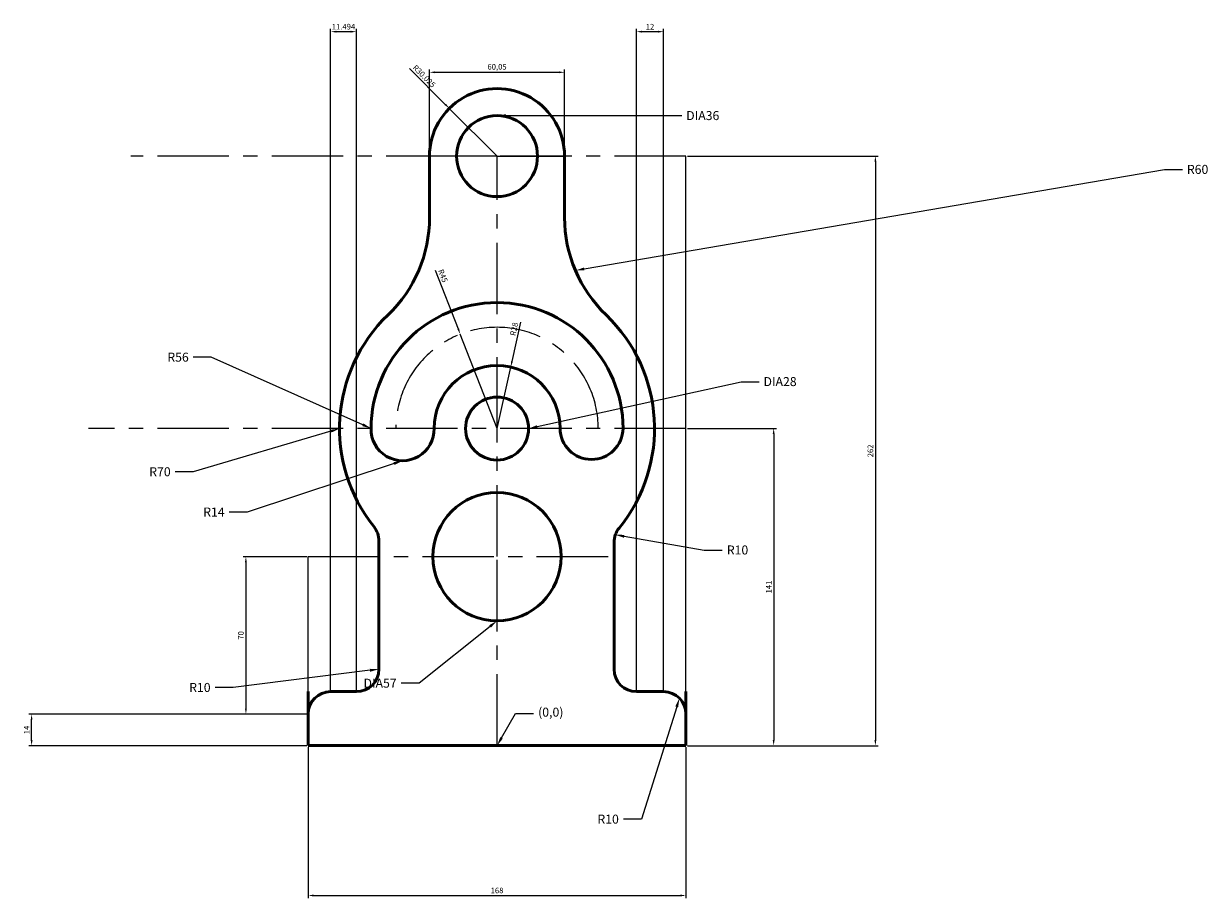
# Model space of a CAD drawing. Units: millimetres. Extents: x 2245 to 2771, y 1191 to 1580.
import ezdxf
from ezdxf import colors
from ezdxf.entities.mleader import LeaderData, LeaderLine
from ezdxf.math import Vec2, Vec3

# ---------------------------------------------------------------- set-up
doc = ezdxf.new("R2010")
doc.units = ezdxf.units.MM
doc.linetypes.add('CENTER', pattern=[50.8, 31.75, -6.35, 6.35, -6.35])
for name, color, linetype, lineweight in [('M-CNTR', 4, 'CENTER', 18), ('M-CONS', 8, 'Continuous', 13), ('M-DIMS', 2, 'Continuous', 25), ('M-OUTL', 7, 'Continuous', 50), ('M-TEXT', 7, 'Continuous', 25)]:
    doc.layers.add(name, color=color, linetype=linetype, lineweight=lineweight)
doc.styles.get("Standard").update_dxf_attribs({"font": 'arial.ttf'})
doc.dimstyles.new('ISO-25', dxfattribs={"dimtxt": 2.5, "dimasz": 2.5, "dimexe": 1.25, "dimexo": 0.625, "dimtad": 1, "dimtxsty": 'Standard', "dimcen": 2.5, "dimadec": 0, "dimazin": 0, "dimtfac": 1, "dimtmove": 0, "dimatfit": 3, "dimfxl": 1, "dimarcsym": 0})

# ---------------------------------------------------------------- blocks, each defined once
blk = doc.blocks.new('*D1')
at = {"layer": 'Defpoints', "color": 0, "transparency": 16777216}
for p in [(2485.25, 1558.14), (2425.2, 1520.84), (2485.25, 1520.87)]:
    blk.add_point(p, dxfattribs=at)
at = {"layer": 'M-DIMS', "color": 0, "lineweight": -2, "transparency": 16777216}
for p, q in [((2425.2, 1521.47), (2425.2, 1559.39)), ((2485.25, 1521.5), (2485.25, 1559.39)), ((2427.7, 1558.14), (2482.75, 1558.14))]:
    blk.add_line(p, q, dxfattribs=at)
at = {"layer": 'M-DIMS', "color": 0, "transparency": 16777216}
for points in [[(2427.7, 1558.56), (2427.7, 1557.73), (2425.2, 1558.14)], [(2482.75, 1558.56), (2482.75, 1557.73), (2485.25, 1558.14)]]:
    blk.add_solid(points, dxfattribs=at)
at = {"layer": 'M-DIMS', "color": 0, "transparency": 16777216, "insert": (2455.23, 1560.27), "char_height": 2.5, "attachment_point": 5}
blk.add_mtext('60,05', dxfattribs=at)
blk = doc.blocks.new('*D2')
at = {"layer": 'Defpoints', "color": 0, "transparency": 16777216}
for p in [(2539.23, 1520.87), (2539.23, 1258.87), (2623.43, 1258.87)]:
    blk.add_point(p, dxfattribs=at)
at = {"layer": 'M-DIMS', "color": 0, "lineweight": -2, "transparency": 16777216}
for p, q in [((2539.85, 1520.87), (2624.68, 1520.87)), ((2623.43, 1518.37), (2623.43, 1261.37)), ((2539.85, 1258.87), (2624.68, 1258.87))]:
    blk.add_line(p, q, dxfattribs=at)
at = {"layer": 'M-DIMS', "color": 0, "transparency": 16777216}
for points in [[(2623.01, 1518.37), (2623.85, 1518.37), (2623.43, 1520.87)], [(2623.01, 1261.37), (2623.85, 1261.37), (2623.43, 1258.87)]]:
    blk.add_solid(points, dxfattribs=at)
at = {"layer": 'M-DIMS', "color": 0, "transparency": 16777216, "insert": (2621.53, 1389.87), "char_height": 2.5, "attachment_point": 5, "rotation": 90}
blk.add_mtext('262', dxfattribs=at)
blk = doc.blocks.new('*D3')
at = {"layer": 'Defpoints', "color": 0, "transparency": 16777216}
for p in [(2371.23, 1342.87), (2343.58, 1272.87), (2371.23, 1272.87)]:
    blk.add_point(p, dxfattribs=at)
at = {"layer": 'M-DIMS', "color": 0, "lineweight": -2, "transparency": 16777216}
for p, q in [((2370.6, 1342.87), (2342.33, 1342.87)), ((2343.58, 1340.37), (2343.58, 1275.37)), ((2370.6, 1272.87), (2342.33, 1272.87))]:
    blk.add_line(p, q, dxfattribs=at)
at = {"layer": 'M-DIMS', "color": 0, "transparency": 16777216}
for points in [[(2343.17, 1340.37), (2344, 1340.37), (2343.58, 1342.87)], [(2343.17, 1275.37), (2344, 1275.37), (2343.58, 1272.87)]]:
    blk.add_solid(points, dxfattribs=at)
at = {"layer": 'M-DIMS', "color": 0, "transparency": 16777216, "insert": (2341.68, 1307.87), "char_height": 2.5, "attachment_point": 5, "rotation": 90}
blk.add_mtext('70', dxfattribs=at)
blk = doc.blocks.new('*D4')
at = {"layer": 'Defpoints', "color": 0, "transparency": 16777216}
for p in [(2539.23, 1399.87), (2539.23, 1258.87), (2578.21, 1258.87)]:
    blk.add_point(p, dxfattribs=at)
at = {"layer": 'M-DIMS', "color": 0, "lineweight": -2, "transparency": 16777216}
for p, q in [((2539.85, 1399.87), (2579.46, 1399.87)), ((2578.21, 1397.37), (2578.21, 1261.37)), ((2539.85, 1258.87), (2579.46, 1258.87))]:
    blk.add_line(p, q, dxfattribs=at)
at = {"layer": 'M-DIMS', "color": 0, "transparency": 16777216}
for points in [[(2577.79, 1397.37), (2578.62, 1397.37), (2578.21, 1399.87)], [(2577.79, 1261.37), (2578.62, 1261.37), (2578.21, 1258.87)]]:
    blk.add_solid(points, dxfattribs=at)
at = {"layer": 'M-DIMS', "color": 0, "transparency": 16777216, "insert": (2576.33, 1329.37), "char_height": 2.5, "attachment_point": 5, "rotation": 90}
blk.add_mtext('141', dxfattribs=at)
blk = doc.blocks.new('*D5')
at = {"layer": 'Defpoints', "color": 0, "transparency": 16777216}
for p in [(2371.23, 1258.87), (2539.23, 1258.87), (2539.23, 1192.29)]:
    blk.add_point(p, dxfattribs=at)
at = {"layer": 'M-DIMS', "color": 0, "lineweight": -2, "transparency": 16777216}
for p, q in [((2371.23, 1258.25), (2371.23, 1191.04)), ((2539.23, 1258.25), (2539.23, 1191.04)), ((2373.73, 1192.29), (2536.73, 1192.29))]:
    blk.add_line(p, q, dxfattribs=at)
at = {"layer": 'M-DIMS', "color": 0, "transparency": 16777216}
for points in [[(2373.73, 1192.7), (2373.73, 1191.87), (2371.23, 1192.29)], [(2536.73, 1192.7), (2536.73, 1191.87), (2539.23, 1192.29)]]:
    blk.add_solid(points, dxfattribs=at)
at = {"layer": 'M-DIMS', "color": 0, "transparency": 16777216, "insert": (2455.23, 1194.19), "char_height": 2.5, "attachment_point": 5}
blk.add_mtext('168', dxfattribs=at)
blk = doc.blocks.new('*D6')
at = {"layer": 'Defpoints', "color": 0, "transparency": 16777216}
for p in [(2248.31, 1272.87), (2371.23, 1272.87), (2371.23, 1258.87)]:
    blk.add_point(p, dxfattribs=at)
at = {"layer": 'M-DIMS', "color": 0, "lineweight": -2, "transparency": 16777216}
for p, q in [((2370.6, 1272.87), (2247.06, 1272.87)), ((2248.31, 1261.37), (2248.31, 1270.37)), ((2370.6, 1258.87), (2247.06, 1258.87))]:
    blk.add_line(p, q, dxfattribs=at)
at = {"layer": 'M-DIMS', "color": 0, "transparency": 16777216}
for points in [[(2247.9, 1270.37), (2248.73, 1270.37), (2248.31, 1272.87)], [(2247.9, 1261.37), (2248.73, 1261.37), (2248.31, 1258.87)]]:
    blk.add_solid(points, dxfattribs=at)
at = {"layer": 'M-DIMS', "color": 0, "transparency": 16777216, "insert": (2246.43, 1265.87), "char_height": 2.5, "attachment_point": 5, "rotation": 90}
blk.add_mtext('14', dxfattribs=at)
blk = doc.blocks.new('*D7')
at = {"layer": 'Defpoints', "color": 0, "transparency": 16777216}
for p in [(2392.72, 1576.2), (2381.23, 1282.87), (2392.72, 1282.87)]:
    blk.add_point(p, dxfattribs=at)
at = {"layer": 'M-DIMS', "color": 0, "lineweight": -2, "transparency": 16777216}
for p, q in [((2381.23, 1283.5), (2381.23, 1577.45)), ((2383.73, 1576.2), (2390.22, 1576.2)), ((2392.72, 1283.5), (2392.72, 1577.45))]:
    blk.add_line(p, q, dxfattribs=at)
at = {"layer": 'M-DIMS', "color": 0, "transparency": 16777216}
for points in [[(2383.73, 1576.62), (2383.73, 1575.78), (2381.23, 1576.2)], [(2390.22, 1576.62), (2390.22, 1575.78), (2392.72, 1576.2)]]:
    blk.add_solid(points, dxfattribs=at)
at = {"layer": 'M-DIMS', "color": 0, "transparency": 16777216, "insert": (2386.97, 1578.1), "char_height": 2.5, "attachment_point": 5}
blk.add_mtext('11.494', dxfattribs=at)
blk = doc.blocks.new('*D8')
at = {"layer": 'Defpoints', "color": 0, "transparency": 16777216}
for p in [(2529.23, 1576.2), (2517.23, 1282.87), (2529.23, 1282.87)]:
    blk.add_point(p, dxfattribs=at)
at = {"layer": 'M-DIMS', "color": 0, "lineweight": -2, "transparency": 16777216}
for p, q in [((2517.23, 1283.5), (2517.23, 1577.45)), ((2519.73, 1576.2), (2526.73, 1576.2)), ((2529.23, 1283.5), (2529.23, 1577.45))]:
    blk.add_line(p, q, dxfattribs=at)
at = {"layer": 'M-DIMS', "color": 0, "transparency": 16777216}
for points in [[(2519.73, 1576.62), (2519.73, 1575.78), (2517.23, 1576.2)], [(2526.73, 1576.62), (2526.73, 1575.78), (2529.23, 1576.2)]]:
    blk.add_solid(points, dxfattribs=at)
at = {"layer": 'M-DIMS', "color": 0, "transparency": 16777216, "insert": (2523.23, 1578.08), "char_height": 2.5, "attachment_point": 5}
blk.add_mtext('12', dxfattribs=at)
blk = doc.blocks.new('*D9')
at = {"layer": 'Defpoints', "color": 0, "transparency": 16777216}
for p in [(2461.3, 1427.13), (2455.23, 1399.8)]:
    blk.add_point(p, dxfattribs=at)
at = {"layer": 'M-DIMS', "color": 0, "lineweight": -2, "transparency": 16777216}
for p, q in [((2465.73, 1447.06), (2461.84, 1429.57)), ((2455.23, 1399.8), (2461.3, 1427.13))]:
    blk.add_line(p, q, dxfattribs=at)
at = {"layer": 'M-DIMS', "color": 0, "transparency": 16777216}
blk.add_solid([(2461.44, 1429.66), (2462.25, 1429.48), (2461.3, 1427.13)], dxfattribs=at)
at = {"layer": 'M-DIMS', "color": 0, "transparency": 16777216, "insert": (2463.09, 1443.94), "char_height": 2.5, "attachment_point": 5, "rotation": 77.4746}
blk.add_mtext('R28', dxfattribs=at)
blk = doc.blocks.new('*D10')
at = {"layer": 'Defpoints', "color": 0, "transparency": 16777216}
for p in [(2438.9, 1441.73), (2455.23, 1399.8)]:
    blk.add_point(p, dxfattribs=at)
at = {"layer": 'M-DIMS', "color": 0, "lineweight": -2, "transparency": 16777216}
for p, q in [((2427.79, 1470.27), (2437.99, 1444.06)), ((2455.23, 1399.8), (2438.9, 1441.73))]:
    blk.add_line(p, q, dxfattribs=at)
at = {"layer": 'M-DIMS', "color": 0, "transparency": 16777216}
blk.add_solid([(2438.38, 1444.21), (2437.6, 1443.91), (2438.9, 1441.73)], dxfattribs=at)
at = {"layer": 'M-DIMS', "color": 0, "transparency": 16777216, "insert": (2430.87, 1467.58), "char_height": 2.5, "attachment_point": 5, "rotation": 291.276}
blk.add_mtext('R45', dxfattribs=at)
blk = doc.blocks.new('*D11')
at = {"layer": 'Defpoints', "color": 0, "transparency": 16777216}
for p in [(2434, 1542.1), (2455.23, 1520.87)]:
    blk.add_point(p, dxfattribs=at)
at = {"layer": 'M-DIMS', "color": 0, "lineweight": -2, "transparency": 16777216}
for p, q in [((2416.29, 1559.8), (2432.23, 1543.87)), ((2455.23, 1520.87), (2434, 1542.1))]:
    blk.add_line(p, q, dxfattribs=at)
at = {"layer": 'M-DIMS', "color": 0, "transparency": 16777216}
blk.add_solid([(2432.52, 1544.17), (2431.93, 1543.58), (2434, 1542.1)], dxfattribs=at)
at = {"layer": 'M-DIMS', "color": 0, "transparency": 16777216, "insert": (2422.6, 1556.19), "char_height": 2.5, "attachment_point": 5, "rotation": 315.0026}
blk.add_mtext('R30.025', dxfattribs=at)

msp = doc.modelspace()

# ---------------------------------------------------------------- linework, layer by layer
at = {"layer": 'M-CNTR'}
for p, q in [((2539.2281, 1520.8738), (2292.4454, 1520.8738)), ((2455.2281, 1520.8738), (2425.2281, 1520.8738)), ((2455.2281, 1399.7988), (2455.2281, 1520.8738)), ((2455.2281, 1520.8738), (2485.2281, 1520.8738)), ((2539.2281, 1399.8738), (2273.6132, 1399.8738)), ((2455.2281, 1342.8738), (2455.2281, 1399.7988)), ((2371.2281, 1342.8738), (2507.2281, 1342.8738)), ((2455.2281, 1258.8738), (2455.2281, 1342.8738))]:
    msp.add_line(p, q, dxfattribs=at)
msp.add_arc((2455.2281, 1399.7988), 45, 0.095576, 179.904424, dxfattribs=at)
at = {"layer": 'M-CONS'}
for p, q in [((2425.2281, 1520.8738), (2425.2281, 1522.0872)), ((2485.2281, 1520.8738), (2485.2281, 1522.0872)), ((2539.2281, 1258.8738), (2539.2281, 1520.8738)), ((2539.2281, 1282.8738), (2539.2281, 1399.8738)), ((2371.2281, 1282.8738), (2371.2281, 1342.8738)), ((2371.2281, 1258.8738), (2455.2281, 1258.8738))]:
    msp.add_line(p, q, dxfattribs=at)
at = {"layer": 'M-OUTL'}
for p, q in [((2425.2035, 1520.8738), (2425.218, 1493.6293)), ((2485.2526, 1520.8738), (2485.2526, 1493.5835)), ((2402.7217, 1299.1162), (2402.7217, 1349.8693)), ((2507.2281, 1303.5728), (2507.2281, 1349.2419)), ((2507.2281, 1292.8738), (2507.2281, 1303.5728)), ((2402.7217, 1292.8738), (2402.7217, 1299.1162)), ((2371.2281, 1282.8738), (2371.2281, 1258.8738)), ((2392.7217, 1282.8738), (2381.2281, 1282.8738)), ((2529.2281, 1282.8738), (2517.2281, 1282.8738)), ((2539.2281, 1258.8738), (2539.2281, 1282.8738)), ((2371.2281, 1258.8738), (2539.2281, 1258.8738))]:
    msp.add_line(p, q, dxfattribs=at)
for centre, radius in [((2455.2281, 1520.8738), 18), ((2455.2281, 1520.8738), 18), ((2455.2281, 1520.8738), 18), ((2455.2281, 1520.8738), 18), ((2455.2281, 1399.7988), 14), ((2455.2281, 1342.8738), 28.5)]:
    msp.add_circle(centre, radius, dxfattribs=at)
for centre, radius, start, end in [((2455.2281, 1520.8738), 30.0245, 0, 180.060794), ((2365.218, 1493.5974), 60, 313.81921, 0.030397), ((2545.2526, 1493.5835), 60, 180, 226.171955), ((2455.2281, 1399.7988), 56, 0.076802, 179.923198), ((2455.2281, 1399.7988), 70, 133.81921, 218.617507), ((2455.2281, 1399.7988), 70, 320.805033, 46.171955), ((2455.2281, 1399.7988), 28, 0.153605, 179.846395), ((2413.2282, 1399.5044), 14.0049, 178.488517, 1.511483), ((2497.228, 1400.0838), 14.0016, 180.859229, 359.140771), ((2392.7217, 1349.8693), 10, 0, 38.617507), ((2517.2281, 1349.2419), 10, 140.805033, 180), ((2392.7217, 1292.8738), 10, 270, 0), ((2517.2281, 1292.8738), 10, 180, 270), ((2381.2281, 1272.8738), 10, 90, 180), ((2529.2281, 1272.8738), 10, 0, 90)]:
    msp.add_arc(centre, radius, start, end, dxfattribs=at)

# ---------------------------------------------------------------- dimensions: what is measured, and where the dimension line sits
at = {"layer": 'M-DIMS'}
for base, p1, p2, override, picture, middle in [((2392.7217, 1576.1984), (2381.2281, 1282.8738), (2392.7217, 1282.8738), {"dimdec": 3, "dimlfac": 1, "dimrnd": 0, "dimzin": 0, "dimdsep": 46, "dimlunit": 2}, '*D7', (2386.9749, 1578.0998)), ((2529.2281, 1576.1984), (2517.2281, 1282.8738), (2529.2281, 1282.8738), {"dimdec": 0, "dimlfac": 1, "dimrnd": 0, "dimzin": 0, "dimdsep": 46, "dimlunit": 2}, '*D8', (2523.2281, 1578.0785)), ((2485.2526, 1558.1445), (2425.2036, 1520.842), (2485.2526, 1520.8738), {"dimclrd": 0, "dimclre": 0, "dimclrt": 0}, '*D1', (2455.2281, 1560.2719)), ((2539.2281, 1192.2879), (2371.2281, 1258.8738), (2539.2281, 1258.8738), {"dimclrd": 0, "dimclre": 0, "dimclrt": 0}, '*D5', (2455.2281, 1194.1893))]:
    dim = msp.add_linear_dim(base=base, p1=p1, p2=p2, dimstyle='ISO-25', override=override, dxfattribs=at)
    dim.commit()
    dim.dimension.update_dxf_attribs({"geometry": picture, "text_midpoint": middle})
for center, mpoint, override, picture, middle in [((2455.2281, 1520.8738), (2433.9966, 1542.1034), {"dimdec": 3, "dimlfac": 1, "dimrnd": 0, "dimzin": 0, "dimdsep": 46, "dimlunit": 2}, '*D11', (2421.2577, 1554.8412)), ((2455.2281, 1399.7988), (2438.8993, 1441.7317), {"dimdec": 0, "dimlfac": 1, "dimrnd": 0, "dimzin": 0, "dimdsep": 46, "dimlunit": 2}, '*D10', (2429.1021, 1466.8915)), ((2455.2281, 1399.7988), (2461.3005, 1427.1324), {"dimdec": 0, "dimlfac": 1, "dimrnd": 0, "dimzin": 0, "dimdsep": 46, "dimlunit": 2}, '*D9', (2464.944, 1443.5325))]:
    dim = msp.add_radius_dim(center=center, mpoint=mpoint, dimstyle='ISO-25', override=override, dxfattribs=at)
    dim.commit()
    dim.dimension.update_dxf_attribs({"geometry": picture, "text_midpoint": middle, "dimtype": 164})
for base, p1, p2, override, picture, middle in [((2623.429, 1258.8738), (2539.2281, 1520.8738), (2539.2281, 1258.8738), {"dimclrd": 0, "dimclre": 0, "dimclrt": 0}, '*D2', (2621.5275, 1389.8738)), ((2578.2071, 1258.8738), (2539.2281, 1399.8738), (2539.2281, 1258.8738), {"dimclrd": 0, "dimclre": 0, "dimclrt": 0}, '*D4', (2576.327, 1329.3738)), ((2343.5849, 1272.8738), (2371.2281, 1342.8738), (2371.2281, 1272.8738), {"dimclrd": 0, "dimclre": 0, "dimclrt": 0}, '*D3', (2341.6835, 1307.8738)), ((2248.3132, 1272.8738), (2371.2281, 1258.8738), (2371.2281, 1272.8738), {"dimdec": 0, "dimlfac": 1, "dimrnd": 0, "dimzin": 0, "dimdsep": 46, "dimlunit": 2}, '*D6', (2246.4331, 1265.8738))]:
    dim = msp.add_linear_dim(base=base, p1=p1, p2=p2, angle=90, dimstyle='ISO-25', override=override, dxfattribs=at)
    dim.commit()
    dim.dimension.update_dxf_attribs({"geometry": picture, "text_midpoint": middle})

# ---------------------------------------------------------------- leaders
ml = msp.add_multileader_mtext('Standard', dxfattribs=at)
ml.set_content('DIA36', color=256)
ml.set_leader_properties()
ml.build(insert=Vec2(0, 0))
ctx = ml.context
ctx.base_point, ctx.plane_origin = Vec3(2537.3285, 1538.8738), Vec3(2455.2281, 1538.8738)
notes = []
notes.append((ctx, [(0, (1, 1, 0), (2529.3285, 1538.8738), (1, 0), 8, [(0, [(2455.2281, 1538.8738)], 0, [])])]))
ctx.mtext.insert, ctx.mtext.flow_direction = Vec3(2539.3285, 1540.9093), 5
ml = msp.add_multileader_mtext('Standard', dxfattribs=at)
ml.set_content('R60', color=256)
ml.set_leader_properties()
ml.build(insert=Vec2(0, 0))
ctx = ml.context
ctx.base_point, ctx.plane_origin = Vec3(2759.9146, 1514.9556), Vec3(2490.0576, 1470.0568)
notes.append((ctx, [(0, (1, 1, 0), (2751.9146, 1514.9556), (1, 0), 8, [(0, [(2490.0576, 1470.0568)], 0, [])])]))
ctx.mtext.insert, ctx.mtext.flow_direction = Vec3(2761.9146, 1516.9897), 5
ml = msp.add_multileader_mtext('Standard', dxfattribs=at)
ml.set_content('R56', color=256)
ml.set_leader_properties()
ml.build(insert=Vec2(0, 0))
ctx = ml.context
ctx.base_point, ctx.plane_origin = Vec3(2306.6285, 1431.5074), Vec3(2399.2281, 1399.8738)
ctx.text_align_type = 2
notes.append((ctx, [(0, (1, 1, 0), (2328.1837, 1431.5074), (-1, 0), 8, [(0, [(2399.2281, 1399.8738)], 0, [])])]))
ctx.mtext.insert, ctx.mtext.alignment, ctx.mtext.flow_direction = Vec3(2318.1837, 1433.5415), 3, 5
ml = msp.add_multileader_mtext('Standard', dxfattribs=at)
ml.set_content('DIA28', color=256)
ml.set_leader_properties()
ml.build(insert=Vec2(0, 0))
ctx = ml.context
ctx.base_point, ctx.plane_origin = Vec3(2571.693, 1420.6464), Vec3(2469.2281, 1399.7988)
notes.append((ctx, [(0, (1, 1, 0), (2563.693, 1420.6464), (1, 0), 8, [(0, [(2469.2281, 1399.7988)], 0, [])])]))
ctx.mtext.insert, ctx.mtext.flow_direction = Vec3(2573.693, 1422.6805), 5
ml = msp.add_multileader_mtext('Standard', dxfattribs=at)
ml.set_content('R70', color=256)
ml.set_leader_properties()
ml.build(insert=Vec2(0, 0))
ctx = ml.context
ctx.base_point, ctx.plane_origin = Vec3(2298.5806, 1380.5708), Vec3(2385.2281, 1399.7988)
ctx.text_align_type = 2
notes.append((ctx, [(0, (1, 1, 0), (2320.125, 1380.5708), (-1, 0), 8, [(0, [(2385.2281, 1399.7988)], 0, [])])]))
ctx.mtext.insert, ctx.mtext.alignment, ctx.mtext.flow_direction = Vec3(2310.125, 1382.6049), 3, 5
ml = msp.add_multileader_mtext('Standard', dxfattribs=at)
ml.set_content('R14', color=256)
ml.set_leader_properties()
ml.build(insert=Vec2(0, 0))
ctx = ml.context
ctx.base_point, ctx.plane_origin = Vec3(2322.5843, 1362.7209), Vec3(2413.2282, 1385.4995)
ctx.text_align_type = 2
notes.append((ctx, [(0, (1, 1, 0), (2344.1259, 1362.7209), (-1, 0), 8, [(0, [(2413.2282, 1385.4995)], 0, [])])]))
ctx.mtext.insert, ctx.mtext.alignment, ctx.mtext.flow_direction = Vec3(2334.1259, 1364.7209), 3, 5
ml = msp.add_multileader_mtext('Standard', dxfattribs=at)
ml.set_content('R10', color=256)
ml.set_leader_properties()
ml.build(insert=Vec2(0, 0))
ctx = ml.context
ctx.base_point, ctx.plane_origin = Vec3(2555.3828, 1345.8089), Vec3(2507.8074, 1352.596)
notes.append((ctx, [(0, (1, 1, 0), (2547.3828, 1345.8089), (1, 0), 8, [(0, [(2507.8074, 1352.596)], 0, [])])]))
ctx.mtext.insert, ctx.mtext.flow_direction = Vec3(2557.3828, 1347.843), 5
ml = msp.add_multileader_mtext('Standard', dxfattribs=at)
ml.set_content('DIA57', color=256)
ml.set_leader_properties()
ml.build(insert=Vec2(0, 0))
ctx = ml.context
ctx.base_point, ctx.plane_origin = Vec3(2393.7576, 1286.6197), Vec3(2455.2281, 1314.3738)
ctx.text_align_type = 2
notes.append((ctx, [(0, (1, 1, 0), (2420.6035, 1286.6197), (-1, 0), 8, [(0, [(2455.2281, 1314.3738)], 0, [])])]))
ctx.mtext.insert, ctx.mtext.alignment, ctx.mtext.flow_direction = Vec3(2410.6035, 1288.6538), 3, 5
ml = msp.add_multileader_mtext('Standard', dxfattribs=at)
ml.set_content('R10', color=256)
ml.set_leader_properties()
ml.build(insert=Vec2(0, 0))
ctx = ml.context
ctx.base_point, ctx.plane_origin = Vec3(2316.3319, 1284.7195), Vec3(2402.7217, 1292.8738)
ctx.text_align_type = 2
notes.append((ctx, [(0, (1, 1, 0), (2337.8763, 1284.7195), (-1, 0), 8, [(0, [(2402.7217, 1292.8738)], 0, [])])]))
ctx.mtext.insert, ctx.mtext.alignment, ctx.mtext.flow_direction = Vec3(2327.8763, 1286.7536), 3, 5
ml = msp.add_multileader_mtext('Standard', dxfattribs=at)
ml.set_content('R10', color=256)
ml.set_leader_properties()
ml.build(insert=Vec2(0, 0))
ctx = ml.context
ctx.base_point, ctx.plane_origin = Vec3(2497.8385, 1226.1833), Vec3(2536.2991, 1279.9449)
ctx.text_align_type = 2
notes.append((ctx, [(0, (1, 1, 0), (2519.3828, 1226.1833), (-1, 0), 8, [(0, [(2536.2991, 1279.9449)], 0, [])])]))
ctx.mtext.insert, ctx.mtext.alignment, ctx.mtext.flow_direction = Vec3(2509.3828, 1228.2174), 3, 5
at = {"layer": 'M-TEXT'}
ml = msp.add_multileader_mtext('Standard', dxfattribs=at)
ml.set_content('(0,0)', color=256)
ml.set_leader_properties()
ml.build(insert=Vec2(0, 0))
ctx = ml.context
ctx.base_point, ctx.plane_origin = Vec3(2471.4858, 1273.1767), Vec3(2455.2281, 1258.8738)
notes.append((ctx, [(0, (1, 1, 0), (2463.4858, 1273.1767), (1, 0), 8, [(0, [(2455.2281, 1258.8738)], 0, [])])]))
ctx.mtext.insert, ctx.mtext.flow_direction = Vec3(2473.4858, 1275.7647), 5
for ctx, leaders in notes:
    for number, flags, end, landing, length, lines in leaders:
        leader = LeaderData()
        leader.index, (leader.has_last_leader_line, leader.has_dogleg_vector, leader.attachment_direction) = number, flags
        leader.last_leader_point, leader.dogleg_vector, leader.dogleg_length = Vec3(end), Vec3(landing), length
        for number, points, colour, breaks in lines:
            line = LeaderLine()
            line.index, line.vertices, line.color, line.breaks = number, Vec3.list(points), colors.encode_raw_color(colour), breaks
            leader.lines.append(line)
        ctx.leaders.append(leader)

doc.saveas('drawing.dxf')
